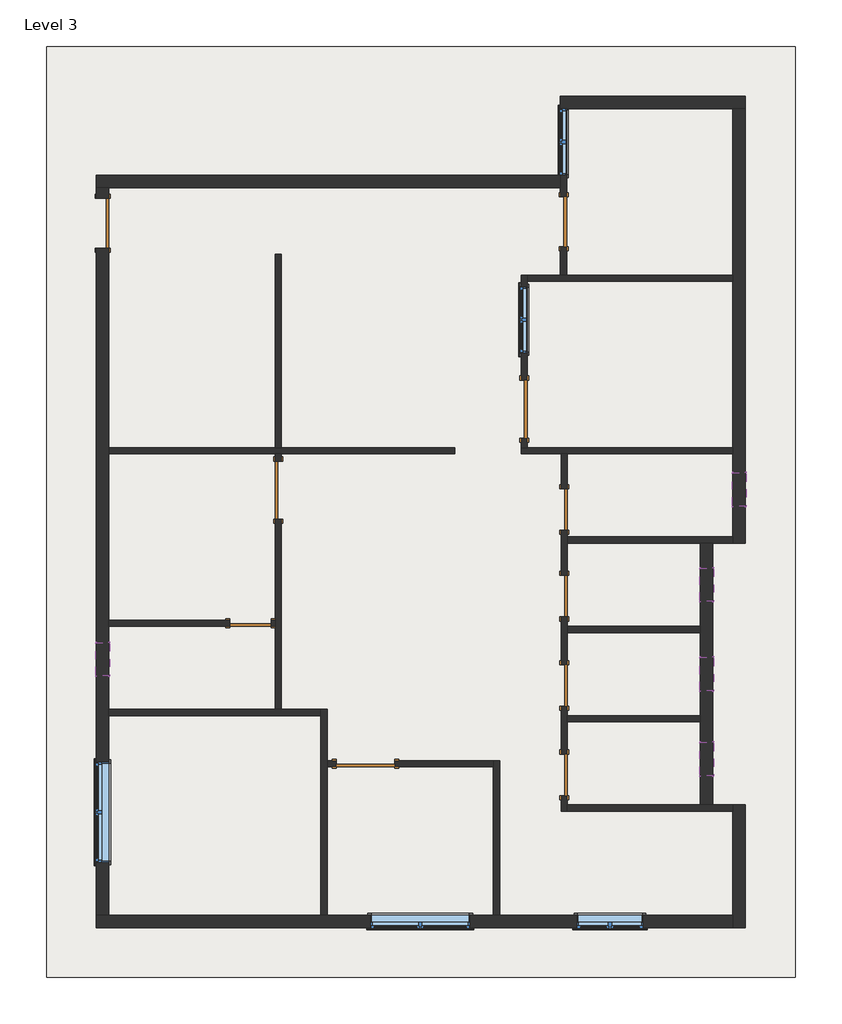
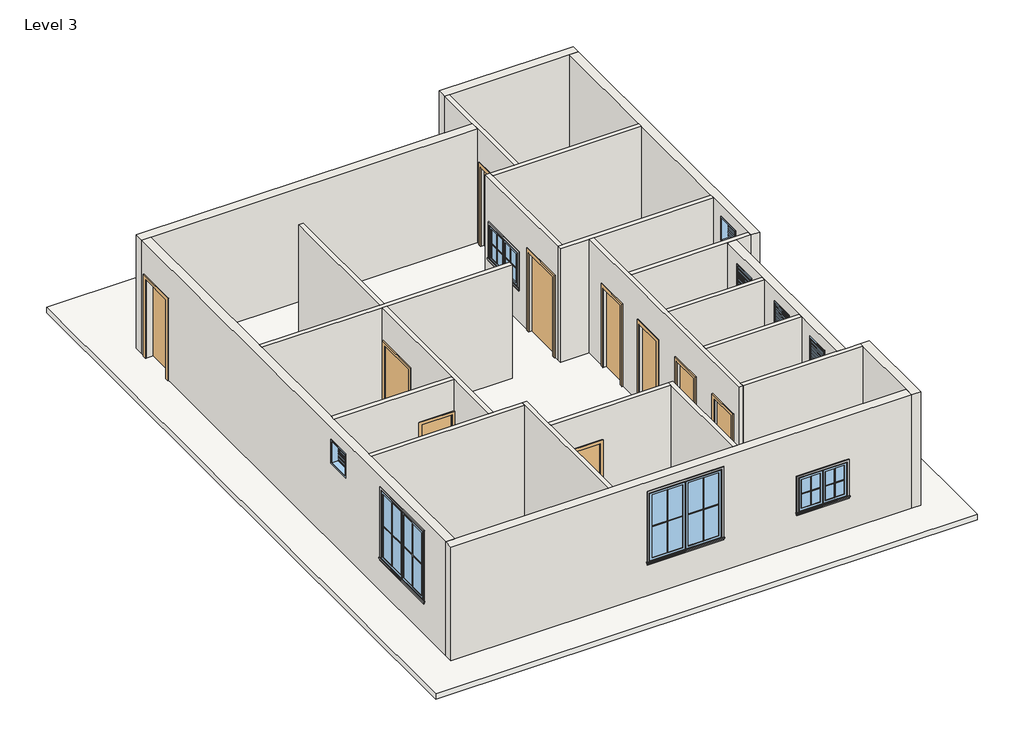
# One storey, incomplete: 23 walls, 20 proxies, 10 doors, 10 windows, 1 roof.
"""IFC4 building model written with IfcOpenShell, lengths in millimetres."""

from ifc_helpers import new_model, si_unit, frame, origin, place, context, project, spatial, polyline, outline, extrude, faceted_brep, transform, mapped, element, save
from components import muntin_pattern_2x2_muntin_pattern_2x2_0a037076, muntin_pattern_2x2_muntin_pattern_2x2_e6f69628, muntin_pattern_2x2_muntin_pattern_2x2_2357e71d, muntin_pattern_2x2_muntin_pattern_2x2_302d8f29, trim_window_exterior_flat_with_sill_b601e94a, trim_window_exterior_flat_with_sill_c4e67c73, trim_window_interior_flat_picture_frame_bfefb25c, trim_window_interior_flat_picture_frame_cf1733af, door_78caadf7, door_214872d5, single_flush_door_3_305aa2a5, single_flush_door_3_a90ba1ad, door_4c162e62, window_casement_double_win_4_c19c33cb, window_casement_double_win_4_2967420f, window_casement_double_win_6_ce442eab, window_f2d8fef0

model = new_model("IFC4")

# Units and contexts
model_context = context("Model", 3, world=origin())
ifc_project = project(units=[si_unit("LENGTHUNIT", "METRE", prefix="MILLI")], contexts=[model_context])

# Site, building, storey
site = spatial("IfcSite", under=ifc_project)
building = spatial("IfcBuilding", under=site)
storey = spatial("IfcBuildingStorey", under=building, Name="Level 3", Elevation=6248.4)

# Proxies
placement = place(None, origin())
muntin_pattern_2x2_muntin_pattern_2x2_shape = muntin_pattern_2x2_muntin_pattern_2x2_0a037076(model_context)
element("IfcBuildingElementProxy", 1, Name="Muntin Pattern_2x2 : Muntin Pattern_2x2", ObjectType="Muntin Pattern_2x2 : Muntin Pattern_2x2", at=placement, inside=storey, context=model_context, shape_type="MappedRepresentation", body=[
    mapped(muntin_pattern_2x2_muntin_pattern_2x2_shape, transform((-7058.058853, -4848.517381, 7232.65), x_axis=(0.0, 1.0, 0.0), y_axis=(-1.0, 0.0, 0.0), z_axis=(0.0, 0.0, 1.0))),
])
element("IfcBuildingElementProxy", 2, Name="Muntin Pattern_2x2 : Muntin Pattern_2x2", ObjectType="Muntin Pattern_2x2 : Muntin Pattern_2x2", at=placement, inside=storey, context=model_context, shape_type="MappedRepresentation", body=[
    mapped(muntin_pattern_2x2_muntin_pattern_2x2_shape, transform((-674.721353, -6497.929881, 7232.65), x_axis=(-1.0, 0.0, 0.0), y_axis=(0.0, -1.0, 0.0), z_axis=(0.0, 0.0, 1.0))),
])
muntin_pattern_2x2_muntin_pattern_2x2_2_shape = muntin_pattern_2x2_muntin_pattern_2x2_e6f69628(model_context)
element("IfcBuildingElementProxy", 3, Name="Muntin Pattern_2x2 : Muntin Pattern_2x2", ObjectType="Muntin Pattern_2x2 : Muntin Pattern_2x2", at=placement, inside=storey, context=model_context, shape_type="MappedRepresentation", body=[
    mapped(muntin_pattern_2x2_muntin_pattern_2x2_2_shape, transform((-7058.058853, -3937.292381, 7232.65), x_axis=(0.0, -1.0, 0.0), y_axis=(1.0, 0.0, 0.0), z_axis=(0.0, 0.0, 1.0))),
])
element("IfcBuildingElementProxy", 4, Name="Muntin Pattern_2x2 : Muntin Pattern_2x2", ObjectType="Muntin Pattern_2x2 : Muntin Pattern_2x2", at=placement, inside=storey, context=model_context, shape_type="MappedRepresentation", body=[
    mapped(muntin_pattern_2x2_muntin_pattern_2x2_2_shape, transform((-1585.946353, -6497.929881, 7232.65), x_axis=(1.0, 0.0, 0.0), y_axis=(0.0, 1.0, 0.0), z_axis=(0.0, 0.0, 1.0))),
])
muntin_pattern_2x2_muntin_pattern_2x2_3_shape = muntin_pattern_2x2_muntin_pattern_2x2_2357e71d(model_context)
element("IfcBuildingElementProxy", 5, Name="Muntin Pattern_2x2 : Muntin Pattern_2x2", ObjectType="Muntin Pattern_2x2 : Muntin Pattern_2x2", at=placement, inside=storey, context=model_context, shape_type="MappedRepresentation", body=[
    mapped(muntin_pattern_2x2_muntin_pattern_2x2_3_shape, transform((2652.678647, -6497.929881, 7232.65), x_axis=(-1.0, 0.0, 0.0), y_axis=(0.0, -1.0, 0.0), z_axis=(0.0, 0.0, 1.0))),
])
element("IfcBuildingElementProxy", 6, Name="Muntin Pattern_2x2 : Muntin Pattern_2x2", ObjectType="Muntin Pattern_2x2 : Muntin Pattern_2x2", at=placement, inside=storey, context=model_context, shape_type="MappedRepresentation", body=[
    mapped(muntin_pattern_2x2_muntin_pattern_2x2_3_shape, transform((727.041147, 4333.582619, 7232.65), x_axis=(0.0, 1.0, 0.0), y_axis=(-1.0, 0.0, 0.0), z_axis=(0.0, 0.0, 1.0))),
])
element("IfcBuildingElementProxy", 7, Name="Muntin Pattern_2x2 : Muntin Pattern_2x2", ObjectType="Muntin Pattern_2x2 : Muntin Pattern_2x2", at=placement, inside=storey, context=model_context, shape_type="MappedRepresentation", body=[
    mapped(muntin_pattern_2x2_muntin_pattern_2x2_3_shape, transform((1450.941147, 7591.132619, 7232.65), x_axis=(0.0, 1.0, 0.0), y_axis=(-1.0, 0.0, 0.0), z_axis=(0.0, 0.0, 1.0))),
])
muntin_pattern_2x2_muntin_pattern_2x2_4_shape = muntin_pattern_2x2_muntin_pattern_2x2_302d8f29(model_context)
element("IfcBuildingElementProxy", 8, Name="Muntin Pattern_2x2 : Muntin Pattern_2x2", ObjectType="Muntin Pattern_2x2 : Muntin Pattern_2x2", at=placement, inside=storey, context=model_context, shape_type="MappedRepresentation", body=[
    mapped(muntin_pattern_2x2_muntin_pattern_2x2_4_shape, transform((2046.253647, -6497.929881, 7232.65), x_axis=(1.0, 0.0, 0.0), y_axis=(0.0, 1.0, 0.0), z_axis=(0.0, 0.0, 1.0))),
])
element("IfcBuildingElementProxy", 9, Name="Muntin Pattern_2x2 : Muntin Pattern_2x2", ObjectType="Muntin Pattern_2x2 : Muntin Pattern_2x2", at=placement, inside=storey, context=model_context, shape_type="MappedRepresentation", body=[
    mapped(muntin_pattern_2x2_muntin_pattern_2x2_4_shape, transform((727.041147, 4940.007619, 7232.65), x_axis=(0.0, -1.0, 0.0), y_axis=(1.0, 0.0, 0.0), z_axis=(0.0, 0.0, 1.0))),
])
element("IfcBuildingElementProxy", 10, Name="Muntin Pattern_2x2 : Muntin Pattern_2x2", ObjectType="Muntin Pattern_2x2 : Muntin Pattern_2x2", at=placement, inside=storey, context=model_context, shape_type="MappedRepresentation", body=[
    mapped(muntin_pattern_2x2_muntin_pattern_2x2_4_shape, transform((1450.941147, 8197.557619, 7232.65), x_axis=(0.0, -1.0, 0.0), y_axis=(1.0, 0.0, 0.0), z_axis=(0.0, 0.0, 1.0))),
])
trim_window_exterior_flat_with_sill_shape = trim_window_exterior_flat_with_sill_b601e94a(model_context)
element("IfcBuildingElementProxy", 11, Name="Trim-Window-Exterior-Flat : with Sill", ObjectType="Trim-Window-Exterior-Flat : with Sill", at=placement, inside=storey, context=model_context, shape_type="MappedRepresentation", body=[
    mapped(trim_window_exterior_flat_with_sill_shape, transform((-7067.583853, -4392.904881, 8991.6), x_axis=(0.0, -1.0, 0.0), y_axis=(0.0, 0.0, 1.0), z_axis=(-1.0, 0.0, 0.0))),
])
element("IfcBuildingElementProxy", 12, Name="Trim-Window-Exterior-Flat : with Sill", ObjectType="Trim-Window-Exterior-Flat : with Sill", at=placement, inside=storey, context=model_context, shape_type="MappedRepresentation", body=[
    mapped(trim_window_exterior_flat_with_sill_shape, transform((-1130.333853, -6507.454881, 8991.6), x_axis=(1.0, 0.0, 0.0), y_axis=(0.0, 0.0, 1.0), z_axis=(0.0, -1.0, 0.0))),
])
trim_window_exterior_flat_with_sill_2_shape = trim_window_exterior_flat_with_sill_c4e67c73(model_context)
element("IfcBuildingElementProxy", 13, Name="Trim-Window-Exterior-Flat : with Sill", ObjectType="Trim-Window-Exterior-Flat : with Sill", at=placement, inside=storey, context=model_context, shape_type="MappedRepresentation", body=[
    mapped(trim_window_exterior_flat_with_sill_2_shape, transform((2349.466147, -6507.454881, 8077.2), x_axis=(1.0, 0.0, 0.0), y_axis=(0.0, 0.0, 1.0), z_axis=(0.0, -1.0, 0.0))),
])
element("IfcBuildingElementProxy", 14, Name="Trim-Window-Exterior-Flat : with Sill", ObjectType="Trim-Window-Exterior-Flat : with Sill", at=placement, inside=storey, context=model_context, shape_type="MappedRepresentation", body=[
    mapped(trim_window_exterior_flat_with_sill_2_shape, transform((717.516147, 4636.795119, 8077.2), x_axis=(0.0, -1.0, 0.0), y_axis=(0.0, 0.0, 1.0), z_axis=(-1.0, 0.0, 0.0))),
])
element("IfcBuildingElementProxy", 15, Name="Trim-Window-Exterior-Flat : with Sill", ObjectType="Trim-Window-Exterior-Flat : with Sill", at=placement, inside=storey, context=model_context, shape_type="MappedRepresentation", body=[
    mapped(trim_window_exterior_flat_with_sill_2_shape, transform((1441.416147, 7894.345119, 8077.2), x_axis=(0.0, -1.0, 0.0), y_axis=(0.0, 0.0, 1.0), z_axis=(-1.0, 0.0, 0.0))),
])
trim_window_interior_flat_picture_frame_shape = trim_window_interior_flat_picture_frame_bfefb25c(model_context)
element("IfcBuildingElementProxy", 16, Name="Trim-Window-Interior-Flat : Picture Frame", ObjectType="Trim-Window-Interior-Flat : Picture Frame", at=placement, inside=storey, context=model_context, shape_type="MappedRepresentation", body=[
    mapped(trim_window_interior_flat_picture_frame_shape, transform((-6838.983853, -4392.904881, 8991.6), x_axis=(0.0, 1.0, 0.0), y_axis=(0.0, 0.0, 1.0), z_axis=(1.0, 0.0, 0.0))),
])
element("IfcBuildingElementProxy", 17, Name="Trim-Window-Interior-Flat : Picture Frame", ObjectType="Trim-Window-Interior-Flat : Picture Frame", at=placement, inside=storey, context=model_context, shape_type="MappedRepresentation", body=[
    mapped(trim_window_interior_flat_picture_frame_shape, transform((-1130.333853, -6278.854881, 8991.6), x_axis=(-1.0, 0.0, 0.0), y_axis=(0.0, 0.0, 1.0), z_axis=(0.0, 1.0, 0.0))),
])
trim_window_interior_flat_picture_frame_2_shape = trim_window_interior_flat_picture_frame_cf1733af(model_context)
element("IfcBuildingElementProxy", 18, Name="Trim-Window-Interior-Flat : Picture Frame", ObjectType="Trim-Window-Interior-Flat : Picture Frame", at=placement, inside=storey, context=model_context, shape_type="MappedRepresentation", body=[
    mapped(trim_window_interior_flat_picture_frame_2_shape, transform((2349.466147, -6278.854881, 8077.2), x_axis=(-1.0, 0.0, 0.0), y_axis=(0.0, 0.0, 1.0), z_axis=(0.0, 1.0, 0.0))),
])
element("IfcBuildingElementProxy", 19, Name="Trim-Window-Interior-Flat : Picture Frame", ObjectType="Trim-Window-Interior-Flat : Picture Frame", at=placement, inside=storey, context=model_context, shape_type="MappedRepresentation", body=[
    mapped(trim_window_interior_flat_picture_frame_2_shape, transform((831.816147, 4636.795119, 8077.2), x_axis=(0.0, 1.0, 0.0), y_axis=(0.0, 0.0, 1.0), z_axis=(1.0, 0.0, 0.0))),
])
element("IfcBuildingElementProxy", 20, Name="Trim-Window-Interior-Flat : Picture Frame", ObjectType="Trim-Window-Interior-Flat : Picture Frame", at=placement, inside=storey, context=model_context, shape_type="MappedRepresentation", body=[
    mapped(trim_window_interior_flat_picture_frame_2_shape, transform((1555.716147, 7894.345119, 8077.2), x_axis=(0.0, 1.0, 0.0), y_axis=(0.0, 0.0, 1.0), z_axis=(1.0, 0.0, 0.0))),
])

# Doors
door_shape = door_78caadf7(model_context)
element("IfcDoor", 21, ObjectType="Single-Flush : 2'6\"", at=placement, inside=storey, context=model_context, shape_type="MappedRepresentation", body=[
    mapped(door_shape, transform((-4241.833853, -925.804881, 6248.4), x_axis=(1.0, 0.0, 0.0), y_axis=(0.0, 1.0, 0.0), z_axis=(0.0, 0.0, 1.0))),
])
door_2_shape = door_214872d5(model_context)
element("IfcDoor", 22, ObjectType="Single-Flush : 2'6\"", at=placement, inside=storey, context=model_context, shape_type="MappedRepresentation", body=[
    mapped(door_2_shape, transform((1511.266147, 1156.995119, 6248.4), x_axis=(0.0, -1.0, 0.0), y_axis=(1.0, 0.0, 0.0), z_axis=(0.0, 0.0, 1.0))),
])
element("IfcDoor", 23, ObjectType="Single-Flush : 2'6\"", at=placement, inside=storey, context=model_context, shape_type="MappedRepresentation", body=[
    mapped(door_2_shape, transform((1511.266147, -430.504881, 6248.4), x_axis=(0.0, -1.0, 0.0), y_axis=(1.0, 0.0, 0.0), z_axis=(0.0, 0.0, 1.0))),
])
element("IfcDoor", 24, ObjectType="Single-Flush : 2'6\"", at=placement, inside=storey, context=model_context, shape_type="MappedRepresentation", body=[
    mapped(door_2_shape, transform((1511.266147, -2068.804881, 6248.4), x_axis=(0.0, -1.0, 0.0), y_axis=(1.0, 0.0, 0.0), z_axis=(0.0, 0.0, 1.0))),
])
element("IfcDoor", 25, ObjectType="Single-Flush : 2'6\"", at=placement, inside=storey, context=model_context, shape_type="MappedRepresentation", body=[
    mapped(door_2_shape, transform((1511.266147, -3707.104881, 6248.4), x_axis=(0.0, -1.0, 0.0), y_axis=(1.0, 0.0, 0.0), z_axis=(0.0, 0.0, 1.0))),
])
single_flush_door_3_shape = single_flush_door_3_305aa2a5(model_context)
element("IfcDoor", 26, ObjectType="Single-Flush : DOOR 3'", at=placement, inside=storey, context=model_context, shape_type="MappedRepresentation", body=[
    mapped(single_flush_door_3_shape, transform((1498.566147, 6433.845119, 6248.4), x_axis=(0.0, 1.0, 0.0), y_axis=(-1.0, 0.0, 0.0), z_axis=(0.0, 0.0, 1.0))),
])
single_flush_door_3_2_shape = single_flush_door_3_a90ba1ad(model_context)
element("IfcDoor", 27, ObjectType="Single-Flush : DOOR 3'", at=placement, inside=storey, context=model_context, shape_type="MappedRepresentation", body=[
    mapped(single_flush_door_3_2_shape, transform((-6953.283853, 6408.445119, 6248.4), x_axis=(0.0, 1.0, 0.0), y_axis=(-1.0, 0.0, 0.0), z_axis=(0.0, 0.0, 1.0))),
])
door_3_shape = door_4c162e62(model_context)
element("IfcDoor", 28, ObjectType="Single-Flush : DOOR 3'6\"", at=placement, inside=storey, context=model_context, shape_type="MappedRepresentation", body=[
    mapped(door_3_shape, transform((-3733.833853, 1512.595119, 6248.4), x_axis=(0.0, 1.0, 0.0), y_axis=(-1.0, 0.0, 0.0), z_axis=(0.0, 0.0, 1.0))),
])
element("IfcDoor", 29, ObjectType="Single-Flush : DOOR 3'6\"", at=placement, inside=storey, context=model_context, shape_type="MappedRepresentation", body=[
    mapped(door_3_shape, transform((774.666147, 2998.495119, 6248.4), x_axis=(0.0, -1.0, 0.0), y_axis=(1.0, 0.0, 0.0), z_axis=(0.0, 0.0, 1.0))),
])
element("IfcDoor", 30, ObjectType="Single-Flush : DOOR 3'6\"", at=placement, inside=storey, context=model_context, shape_type="MappedRepresentation", body=[
    mapped(door_3_shape, transform((-2133.633853, -3503.904881, 6248.4), x_axis=(-1.0, 0.0, 0.0), y_axis=(0.0, -1.0, 0.0), z_axis=(0.0, 0.0, 1.0))),
])

# Roof
element("IfcRoof", 31, ObjectType="Generic - 12\"", at=placement, inside=storey, context=model_context, shape_type="SweptSolid", body=[
    extrude(outline(polyline([(-7981.983853, 9646.945119), (5746.716147, 9646.945119), (5746.716147, -7421.854881), (-7981.983853, -7421.854881), (-7981.983853, 9646.945119)])), frame((0.0, 0.0, 6096.0), z_axis=(0.0, 0.0, 1.0), x_axis=(1.0, 0.0, 0.0)), (0.0, 0.0, 1.0), 152.4),
])

# Walls
element("IfcWall", 32, ObjectType="WALL 4.5\"", at=placement, inside=storey, context=model_context, shape_type="Brep", body=[
    faceted_brep([(-6838.983853, 2179.345119, 6248.4), (-3790.983853, 2179.345119, 6248.4), (-3676.683853, 2179.345119, 6248.4), (-501.683853, 2179.345119, 6248.4), (-501.683853, 2179.345119, 9296.4), (-3676.683853, 2179.345119, 9296.4), (-3790.983853, 2179.345119, 9296.4), (-6838.983853, 2179.345119, 9296.4), (-6838.983853, 2293.645119, 6248.4), (-6838.983853, 2293.645119, 9296.4), (-3790.983853, 2293.645119, 9296.4), (-3676.683853, 2293.645119, 9296.4), (-501.683853, 2293.645119, 9296.4), (-501.683853, 2293.645119, 6248.4), (-3676.683853, 2293.645119, 6248.4), (-3790.983853, 2293.645119, 6248.4)], [[[0, 1, 2, 3, 4, 5, 6, 7]], [[8, 9, 10, 11, 12, 13, 14, 15]], [[3, 2, 1, 0, 8, 15, 14, 13]], [[4, 3, 13, 12]], [[0, 7, 9, 8]], [[7, 6, 5, 4, 12, 11, 10, 9]]]),
])
element("IfcWall", 33, ObjectType="WALL 4.5\"", at=placement, inside=storey, context=model_context, shape_type="Brep", body=[
    faceted_brep([(-2838.483853, -6278.854881, 6248.4), (-2838.483853, -3561.054881, 6248.4), (-2838.483853, -3446.754881, 6248.4), (-2838.483853, -2506.954881, 6248.4), (-2838.483853, -2506.954881, 9296.4), (-2838.483853, -3446.754881, 9296.4), (-2838.483853, -3561.054881, 9296.4), (-2838.483853, -6278.854881, 9296.4), (-2952.783853, -6278.854881, 6248.4), (-2952.783853, -6278.854881, 9296.4), (-2952.783853, -2621.254881, 9296.4), (-2952.783853, -2506.954881, 9296.4), (-2952.783853, -2506.954881, 6248.4), (-2952.783853, -2621.254881, 6248.4)], [[[0, 1, 2, 3, 4, 5, 6, 7]], [[8, 9, 10, 11, 12, 13]], [[3, 2, 1, 0, 8, 13, 12]], [[0, 7, 9, 8]], [[4, 3, 12, 11]], [[7, 6, 5, 4, 11, 10, 9]]]),
])
element("IfcWall", 34, ObjectType="WALL 4.5\"", at=placement, inside=storey, context=model_context, shape_type="Brep", body=[
    faceted_brep([(-2952.783853, -2506.954881, 6248.4), (-3676.683853, -2506.954881, 6248.4), (-3790.983853, -2506.954881, 6248.4), (-6838.983853, -2506.954881, 6248.4), (-6838.983853, -2506.954881, 9296.4), (-3790.983853, -2506.954881, 9296.4), (-3676.683853, -2506.954881, 9296.4), (-2952.783853, -2506.954881, 9296.4), (-2952.783853, -2621.254881, 6248.4), (-2952.783853, -2621.254881, 9296.4), (-6838.983853, -2621.254881, 9296.4), (-6838.983853, -2621.254881, 6248.4)], [[[0, 1, 2, 3, 4, 5, 6, 7]], [[8, 9, 10, 11]], [[3, 2, 1, 0, 8, 11]], [[0, 7, 9, 8]], [[4, 3, 11, 10]], [[7, 6, 5, 4, 10, 9]]]),
])
element("IfcWall", 35, ObjectType="WALL 4.5\"", at=placement, inside=storey, context=model_context, shape_type="SweptSolid", body=[
    extrude(outline(polyline([(8382.0, -3860.833853), (6248.4, -3860.833853), (6248.4, -3790.983853), (9296.4, -3790.983853), (9296.4, -6838.983853), (6248.4, -6838.983853), (6248.4, -4622.833853), (8382.0, -4622.833853), (8382.0, -3860.833853)])), frame((0.0, -982.954881, 0.0), z_axis=(0.0, 1.0, 0.0), x_axis=(0.0, 0.0, 1.0)), (0.0, 0.0, 1.0), 114.3),
])
element("IfcWall", 36, ObjectType="WALL 4.5\"", at=placement, inside=storey, context=model_context, shape_type="Brep", body=[
    faceted_brep([(-3676.683853, 5836.945119, 6248.4), (-3676.683853, 5836.945119, 9296.4), (-3676.683853, 2293.645119, 9296.4), (-3676.683853, 2293.645119, 6248.4), (-3790.983853, 5836.945119, 9296.4), (-3790.983853, 5836.945119, 6248.4), (-3790.983853, 2293.645119, 6248.4), (-3790.983853, 2293.645119, 9296.4)], [[[0, 1, 2, 3]], [[4, 5, 6, 7]], [[5, 0, 3, 6]], [[1, 0, 5, 4]], [[3, 2, 7, 6]], [[1, 4, 7, 2]]]),
    faceted_brep([(-3676.683853, -2506.954881, 9296.4), (-3676.683853, -2506.954881, 6248.4), (-3676.683853, 979.195119, 6248.4), (-3676.683853, 979.195119, 8382.0), (-3676.683853, 2045.995119, 8382.0), (-3676.683853, 2045.995119, 6248.4), (-3676.683853, 2179.345119, 6248.4), (-3676.683853, 2179.345119, 9296.4), (-3790.983853, -2506.954881, 6248.4), (-3790.983853, -2506.954881, 9296.4), (-3790.983853, -982.954881, 9296.4), (-3790.983853, -868.654881, 9296.4), (-3790.983853, 2179.345119, 9296.4), (-3790.983853, 2179.345119, 6248.4), (-3790.983853, 2045.995119, 6248.4), (-3790.983853, 2045.995119, 8382.0), (-3790.983853, 979.195119, 8382.0), (-3790.983853, 979.195119, 6248.4), (-3790.983853, -868.654881, 6248.4), (-3790.983853, -982.954881, 6248.4)], [[[0, 1, 2, 3, 4, 5, 6, 7]], [[8, 9, 10, 11, 12, 13, 14, 15, 16, 17, 18, 19]], [[1, 8, 19, 18, 17, 2]], [[5, 14, 13, 6]], [[1, 0, 9, 8]], [[7, 6, 13, 12]], [[15, 14, 5, 4]], [[16, 15, 4, 3]], [[17, 16, 3, 2]], [[9, 0, 7, 12, 11, 10]]]),
])
element("IfcWall", 37, ObjectType="WALL 4.5\"", at=placement, inside=storey, context=model_context, shape_type="Brep", body=[
    faceted_brep([(4603.716147, 2293.645119, 6248.4), (831.816147, 2293.645119, 6248.4), (717.516147, 2293.645119, 6248.4), (717.516147, 2293.645119, 9296.4), (831.816147, 2293.645119, 9296.4), (4603.716147, 2293.645119, 9296.4), (4603.716147, 2179.345119, 6248.4), (4603.716147, 2179.345119, 9296.4), (1568.416147, 2179.345119, 9296.4), (1454.116147, 2179.345119, 9296.4), (717.516147, 2179.345119, 9296.4), (717.516147, 2179.345119, 6248.4), (1454.116147, 2179.345119, 6248.4), (1568.416147, 2179.345119, 6248.4)], [[[0, 1, 2, 3, 4, 5]], [[6, 7, 8, 9, 10, 11, 12, 13]], [[2, 1, 0, 6, 13, 12, 11]], [[0, 5, 7, 6]], [[3, 2, 11, 10]], [[5, 4, 3, 10, 9, 8, 7]]]),
])
element("IfcWall", 38, ObjectType="WALL 4.5\"", at=placement, inside=storey, context=model_context, shape_type="Brep", body=[
    faceted_brep([(831.816147, 2293.645119, 6248.4), (831.816147, 2465.095119, 6248.4), (831.816147, 2465.095119, 8382.0), (831.816147, 3531.895119, 8382.0), (831.816147, 3531.895119, 6248.4), (831.816147, 5341.645119, 6248.4), (831.816147, 5455.945119, 6248.4), (831.816147, 5455.945119, 9296.4), (831.816147, 5341.645119, 9296.4), (831.816147, 2293.645119, 9296.4), (831.816147, 5246.395119, 8077.2), (831.816147, 5246.395119, 7162.8), (831.816147, 4027.195119, 7162.8), (831.816147, 4027.195119, 8077.2), (717.516147, 2465.095119, 8382.0), (717.516147, 2465.095119, 6248.4), (717.516147, 2293.645119, 6248.4), (717.516147, 2293.645119, 9296.4), (717.516147, 5455.945119, 9296.4), (717.516147, 5455.945119, 6248.4), (717.516147, 3531.895119, 6248.4), (717.516147, 3531.895119, 8382.0), (717.516147, 5246.395119, 8077.2), (717.516147, 4027.195119, 8077.2), (717.516147, 4027.195119, 7162.8), (717.516147, 5246.395119, 7162.8)], [[[0, 1, 2, 3, 4, 5, 6, 7, 8, 9], [10, 11, 12, 13]], [[14, 15, 16, 17, 18, 19, 20, 21], [22, 23, 24, 25]], [[20, 19, 6, 5, 4]], [[16, 15, 1, 0]], [[0, 9, 17, 16]], [[7, 6, 19, 18]], [[11, 10, 22, 25]], [[12, 11, 25, 24]], [[13, 12, 24, 23]], [[10, 13, 23, 22]], [[2, 1, 15, 14]], [[3, 2, 14, 21]], [[4, 3, 21, 20]], [[9, 8, 7, 18, 17]]]),
])
element("IfcWall", 39, ObjectType="WALL 4.5\"", at=placement, inside=storey, context=model_context, shape_type="Brep", body=[
    faceted_brep([(831.816147, 5341.645119, 6248.4), (4603.716147, 5341.645119, 6248.4), (4603.716147, 5341.645119, 9296.4), (831.816147, 5341.645119, 9296.4), (831.816147, 5455.945119, 6248.4), (831.816147, 5455.945119, 9296.4), (1441.416147, 5455.945119, 9296.4), (1555.716147, 5455.945119, 9296.4), (4603.716147, 5455.945119, 9296.4), (4603.716147, 5455.945119, 6248.4), (1555.716147, 5455.945119, 6248.4), (1441.416147, 5455.945119, 6248.4)], [[[0, 1, 2, 3]], [[4, 5, 6, 7, 8, 9, 10, 11]], [[1, 0, 4, 11, 10, 9]], [[0, 3, 5, 4]], [[2, 1, 9, 8]], [[3, 2, 8, 7, 6, 5]]]),
])
element("IfcWall", 40, ObjectType="WALL 4.5\"", at=placement, inside=storey, context=model_context, shape_type="Brep", body=[
    faceted_brep([(1555.716147, 6891.045119, 8382.0), (1555.716147, 6891.045119, 6248.4), (1555.716147, 8503.945119, 6248.4), (1555.716147, 8503.945119, 7162.8), (1555.716147, 7284.745119, 7162.8), (1555.716147, 7284.745119, 8077.2), (1555.716147, 8503.945119, 8077.2), (1555.716147, 8503.945119, 9296.4), (1555.716147, 5455.945119, 9296.4), (1555.716147, 5455.945119, 6248.4), (1555.716147, 5976.645119, 6248.4), (1555.716147, 5976.645119, 8382.0), (1441.416147, 8503.945119, 6248.4), (1441.416147, 7284.745119, 6248.4), (1441.416147, 7056.145119, 6248.4), (1441.416147, 6891.045119, 6248.4), (1441.416147, 6891.045119, 8382.0), (1441.416147, 5976.645119, 8382.0), (1441.416147, 5976.645119, 6248.4), (1441.416147, 5455.945119, 6248.4), (1441.416147, 5455.945119, 9296.4), (1441.416147, 7056.145119, 9296.4), (1441.416147, 7284.745119, 9296.4), (1441.416147, 8503.945119, 9296.4), (1441.416147, 8503.945119, 8077.2), (1441.416147, 7284.745119, 8077.2), (1441.416147, 7284.745119, 7162.8), (1441.416147, 8503.945119, 7162.8)], [[[0, 1, 2, 3, 4, 5, 6, 7, 8, 9, 10, 11]], [[12, 13, 14, 15, 16, 17, 18, 19, 20, 21, 22, 23, 24, 25, 26, 27]], [[10, 9, 19, 18]], [[2, 1, 15, 14, 13, 12]], [[24, 23, 7, 6]], [[12, 27, 3, 2]], [[9, 8, 20, 19]], [[4, 3, 27, 26]], [[5, 4, 26, 25]], [[6, 5, 25, 24]], [[16, 15, 1, 0]], [[17, 16, 0, 11]], [[18, 17, 11, 10]], [[8, 7, 23, 22, 21, 20]]]),
])
element("IfcWall", 41, ObjectType="WALL 4.5\"", at=placement, inside=storey, context=model_context, shape_type="Brep", body=[
    faceted_brep([(4603.716147, 655.345119, 6248.4), (1568.416147, 655.345119, 6248.4), (1568.416147, 655.345119, 9296.4), (4603.716147, 655.345119, 9296.4), (4603.716147, 541.045119, 6248.4), (4603.716147, 541.045119, 9296.4), (4235.416147, 541.045119, 9296.4), (4006.816147, 541.045119, 9296.4), (1568.416147, 541.045119, 9296.4), (1568.416147, 541.045119, 6248.4), (4006.816147, 541.045119, 6248.4), (4235.416147, 541.045119, 6248.4)], [[[0, 1, 2, 3]], [[4, 5, 6, 7, 8, 9, 10, 11]], [[1, 0, 4, 11, 10, 9]], [[0, 3, 5, 4]], [[2, 1, 9, 8]], [[3, 2, 8, 7, 6, 5]]]),
])
element("IfcWall", 42, ObjectType="WALL 4.5\"", at=placement, inside=storey, context=model_context, shape_type="Brep", body=[
    faceted_brep([(1454.116147, -4088.104881, 8382.0), (1454.116147, -4088.104881, 6248.4), (1454.116147, -4373.854881, 6248.4), (1454.116147, -4373.854881, 9296.4), (1454.116147, 2179.345119, 9296.4), (1454.116147, 2179.345119, 6248.4), (1454.116147, 1537.995119, 6248.4), (1454.116147, 1537.995119, 8382.0), (1454.116147, 775.995119, 8382.0), (1454.116147, 775.995119, 6248.4), (1454.116147, -49.504881, 6248.4), (1454.116147, -49.504881, 8382.0), (1454.116147, -811.504881, 8382.0), (1454.116147, -811.504881, 6248.4), (1454.116147, -1687.804881, 6248.4), (1454.116147, -1687.804881, 8382.0), (1454.116147, -2449.804881, 8382.0), (1454.116147, -2449.804881, 6248.4), (1454.116147, -3326.104881, 6248.4), (1454.116147, -3326.104881, 8382.0), (1568.416147, -4373.854881, 6248.4), (1568.416147, -4259.554881, 6248.4), (1568.416147, -4088.104881, 6248.4), (1568.416147, -4088.104881, 8382.0), (1568.416147, -3326.104881, 8382.0), (1568.416147, -3326.104881, 6248.4), (1568.416147, -2735.554881, 6248.4), (1568.416147, -2621.254881, 6248.4), (1568.416147, -2449.804881, 6248.4), (1568.416147, -2449.804881, 8382.0), (1568.416147, -1687.804881, 8382.0), (1568.416147, -1687.804881, 6248.4), (1568.416147, -1097.254881, 6248.4), (1568.416147, -982.954881, 6248.4), (1568.416147, -811.504881, 6248.4), (1568.416147, -811.504881, 8382.0), (1568.416147, -49.504881, 8382.0), (1568.416147, -49.504881, 6248.4), (1568.416147, 541.045119, 6248.4), (1568.416147, 655.345119, 6248.4), (1568.416147, 775.995119, 6248.4), (1568.416147, 775.995119, 8382.0), (1568.416147, 1537.995119, 8382.0), (1568.416147, 1537.995119, 6248.4), (1568.416147, 2179.345119, 6248.4), (1568.416147, 2179.345119, 9296.4), (1568.416147, 655.345119, 9296.4), (1568.416147, 541.045119, 9296.4), (1568.416147, -982.954881, 9296.4), (1568.416147, -1097.254881, 9296.4), (1568.416147, -2621.254881, 9296.4), (1568.416147, -2735.554881, 9296.4), (1568.416147, -4259.554881, 9296.4), (1568.416147, -4373.854881, 9296.4)], [[[0, 1, 2, 3, 4, 5, 6, 7, 8, 9, 10, 11, 12, 13, 14, 15, 16, 17, 18, 19]], [[20, 21, 22, 23, 24, 25, 26, 27, 28, 29, 30, 31, 32, 33, 34, 35, 36, 37, 38, 39, 40, 41, 42, 43, 44, 45, 46, 47, 48, 49, 50, 51, 52, 53]], [[6, 5, 44, 43]], [[10, 9, 40, 39, 38, 37]], [[14, 13, 34, 33, 32, 31]], [[18, 17, 28, 27, 26, 25]], [[2, 1, 22, 21, 20]], [[5, 4, 45, 44]], [[3, 2, 20, 53]], [[41, 40, 9, 8]], [[42, 41, 8, 7]], [[43, 42, 7, 6]], [[35, 34, 13, 12]], [[36, 35, 12, 11]], [[37, 36, 11, 10]], [[29, 28, 17, 16]], [[30, 29, 16, 15]], [[31, 30, 15, 14]], [[23, 22, 1, 0]], [[24, 23, 0, 19]], [[25, 24, 19, 18]], [[4, 3, 53, 52, 51, 50, 49, 48, 47, 46, 45]]]),
])
element("IfcWall", 43, ObjectType="WALL 4.5\"", at=placement, inside=storey, context=model_context, shape_type="Brep", body=[
    faceted_brep([(1568.416147, -4373.854881, 6248.4), (4603.716147, -4373.854881, 6248.4), (4603.716147, -4373.854881, 9296.4), (1568.416147, -4373.854881, 9296.4), (1568.416147, -4259.554881, 6248.4), (1568.416147, -4259.554881, 9296.4), (4006.816147, -4259.554881, 9296.4), (4235.416147, -4259.554881, 9296.4), (4603.716147, -4259.554881, 9296.4), (4603.716147, -4259.554881, 6248.4), (4235.416147, -4259.554881, 6248.4), (4006.816147, -4259.554881, 6248.4)], [[[0, 1, 2, 3]], [[4, 5, 6, 7, 8, 9, 10, 11]], [[1, 0, 4, 11, 10, 9]], [[0, 3, 5, 4]], [[2, 1, 9, 8]], [[3, 2, 8, 7, 6, 5]]]),
])
element("IfcWall", 44, ObjectType="WALL 4.5\"", at=placement, inside=storey, context=model_context, shape_type="SweptSolid", body=[
    extrude(outline(polyline([(4006.816147, -2735.554881), (1568.416147, -2735.554881), (1568.416147, -2621.254881), (4006.816147, -2621.254881), (4006.816147, -2735.554881)])), frame((0.0, 0.0, 6248.4), z_axis=(0.0, 0.0, 1.0), x_axis=(1.0, 0.0, 0.0)), (0.0, 0.0, 1.0), 3048.0),
])
element("IfcWall", 45, ObjectType="WALL 4.5\"", at=placement, inside=storey, context=model_context, shape_type="SweptSolid", body=[
    extrude(outline(polyline([(4006.816147, -1097.254881), (1568.416147, -1097.254881), (1568.416147, -982.954881), (4006.816147, -982.954881), (4006.816147, -1097.254881)])), frame((0.0, 0.0, 6248.4), z_axis=(0.0, 0.0, 1.0), x_axis=(1.0, 0.0, 0.0)), (0.0, 0.0, 1.0), 3048.0),
])
element("IfcWall", 46, ObjectType="WALL 4.5\"", at=placement, inside=storey, context=model_context, shape_type="Brep", body=[
    faceted_brep([(323.816147, -6278.854881, 6248.4), (323.816147, -3446.754881, 6248.4), (323.816147, -3446.754881, 9296.4), (323.816147, -6278.854881, 9296.4), (209.516147, -6278.854881, 6248.4), (209.516147, -6278.854881, 9296.4), (209.516147, -3561.054881, 9296.4), (209.516147, -3446.754881, 9296.4), (209.516147, -3446.754881, 6248.4), (209.516147, -3561.054881, 6248.4)], [[[0, 1, 2, 3]], [[4, 5, 6, 7, 8, 9]], [[1, 0, 4, 9, 8]], [[0, 3, 5, 4]], [[2, 1, 8, 7]], [[3, 2, 7, 6, 5]]]),
])
element("IfcWall", 47, ObjectType="WALL 4.5\"", at=placement, inside=storey, context=model_context, shape_type="SweptSolid", body=[
    extrude(outline(polyline([(6248.4, -2838.483853), (6248.4, -2667.033853), (8382.0, -2667.033853), (8382.0, -1600.233853), (6248.4, -1600.233853), (6248.4, 209.516147), (9296.4, 209.516147), (9296.4, -2838.483853), (6248.4, -2838.483853)])), frame((0.0, -3561.054881, 0.0), z_axis=(0.0, 1.0, 0.0), x_axis=(0.0, 0.0, 1.0)), (0.0, 0.0, 1.0), 114.3),
])
element("IfcWall", 48, ObjectType="WALL 9\"", at=placement, inside=storey, context=model_context, shape_type="Brep", body=[
    faceted_brep([(-7067.583853, 7056.145119, 6248.4), (-6838.983853, 7056.145119, 6248.4), (1441.416147, 7056.145119, 6248.4), (1441.416147, 7056.145119, 9296.4), (-6838.983853, 7056.145119, 9296.4), (-7067.583853, 7056.145119, 9296.4), (-7067.583853, 7284.745119, 6248.4), (-7067.583853, 7284.745119, 9296.4), (1441.416147, 7284.745119, 9296.4), (1441.416147, 7284.745119, 6248.4)], [[[0, 1, 2, 3, 4, 5]], [[6, 7, 8, 9]], [[2, 1, 0, 6, 9]], [[0, 5, 7, 6]], [[3, 2, 9, 8]], [[5, 4, 3, 8, 7]]]),
])
element("IfcWall", 49, ObjectType="WALL 9\"", at=placement, inside=storey, context=model_context, shape_type="Brep", body=[
    faceted_brep([(1441.416147, 8503.945119, 6248.4), (1555.716147, 8503.945119, 6248.4), (4603.716147, 8503.945119, 6248.4), (4832.316147, 8503.945119, 6248.4), (4832.316147, 8503.945119, 9296.4), (4603.716147, 8503.945119, 9296.4), (1555.716147, 8503.945119, 9296.4), (1441.416147, 8503.945119, 9296.4), (1441.416147, 8503.945119, 8077.2), (1441.416147, 8503.945119, 7162.8), (1441.416147, 8732.545119, 6248.4), (1441.416147, 8732.545119, 9296.4), (4832.316147, 8732.545119, 9296.4), (4832.316147, 8732.545119, 6248.4)], [[[0, 1, 2, 3, 4, 5, 6, 7, 8, 9]], [[10, 11, 12, 13]], [[3, 2, 1, 0, 10, 13]], [[4, 3, 13, 12]], [[0, 9, 8, 7, 11, 10]], [[7, 6, 5, 4, 12, 11]]]),
])
element("IfcWall", 50, ObjectType="WALL 9\"", at=placement, inside=storey, context=model_context, shape_type="Brep", body=[
    faceted_brep([(4603.716147, 8503.945119, 6248.4), (4603.716147, 5455.945119, 6248.4), (4603.716147, 5341.645119, 6248.4), (4603.716147, 2293.645119, 6248.4), (4603.716147, 2179.345119, 6248.4), (4603.716147, 655.345119, 6248.4), (4603.716147, 541.045119, 6248.4), (4603.716147, 541.045119, 9296.4), (4603.716147, 655.345119, 9296.4), (4603.716147, 2179.345119, 9296.4), (4603.716147, 2293.645119, 9296.4), (4603.716147, 5341.645119, 9296.4), (4603.716147, 5455.945119, 9296.4), (4603.716147, 8503.945119, 9296.4), (4603.716147, 1830.095119, 8991.6), (4603.716147, 1220.495119, 8991.6), (4603.716147, 1220.495119, 8382.0), (4603.716147, 1830.095119, 8382.0), (4832.316147, 8503.945119, 6248.4), (4832.316147, 8503.945119, 9296.4), (4832.316147, 541.045119, 9296.4), (4832.316147, 541.045119, 6248.4), (4832.316147, 1830.095119, 8991.6), (4832.316147, 1830.095119, 8382.0), (4832.316147, 1220.495119, 8382.0), (4832.316147, 1220.495119, 8991.6)], [[[0, 1, 2, 3, 4, 5, 6, 7, 8, 9, 10, 11, 12, 13], [14, 15, 16, 17]], [[18, 19, 20, 21], [22, 23, 24, 25]], [[6, 5, 4, 3, 2, 1, 0, 18, 21]], [[0, 13, 19, 18]], [[7, 6, 21, 20]], [[23, 22, 14, 17]], [[24, 23, 17, 16]], [[25, 24, 16, 15]], [[22, 25, 15, 14]], [[13, 12, 11, 10, 9, 8, 7, 20, 19]]]),
])
element("IfcWall", 51, ObjectType="WALL 9\"", at=placement, inside=storey, context=model_context, shape_type="Brep", body=[
    faceted_brep([(4006.816147, 541.045119, 6248.4), (4006.816147, -982.954881, 6248.4), (4006.816147, -1097.254881, 6248.4), (4006.816147, -2621.254881, 6248.4), (4006.816147, -2735.554881, 6248.4), (4006.816147, -4259.554881, 6248.4), (4006.816147, -4259.554881, 9296.4), (4006.816147, -2735.554881, 9296.4), (4006.816147, -2621.254881, 9296.4), (4006.816147, -1097.254881, 9296.4), (4006.816147, -982.954881, 9296.4), (4006.816147, 541.045119, 9296.4), (4006.816147, -525.754881, 8991.6), (4006.816147, -525.754881, 8382.0), (4006.816147, 83.845119, 8382.0), (4006.816147, 83.845119, 8991.6), (4006.816147, -2164.054881, 8991.6), (4006.816147, -2164.054881, 8382.0), (4006.816147, -1554.454881, 8382.0), (4006.816147, -1554.454881, 8991.6), (4006.816147, -3719.804881, 8991.6), (4006.816147, -3719.804881, 8382.0), (4006.816147, -3110.204881, 8382.0), (4006.816147, -3110.204881, 8991.6), (4235.416147, 541.045119, 6248.4), (4235.416147, 541.045119, 9296.4), (4235.416147, -4259.554881, 9296.4), (4235.416147, -4259.554881, 6248.4), (4235.416147, -525.754881, 8991.6), (4235.416147, 83.845119, 8991.6), (4235.416147, 83.845119, 8382.0), (4235.416147, -525.754881, 8382.0), (4235.416147, -2164.054881, 8991.6), (4235.416147, -1554.454881, 8991.6), (4235.416147, -1554.454881, 8382.0), (4235.416147, -2164.054881, 8382.0), (4235.416147, -3719.804881, 8991.6), (4235.416147, -3110.204881, 8991.6), (4235.416147, -3110.204881, 8382.0), (4235.416147, -3719.804881, 8382.0)], [[[0, 1, 2, 3, 4, 5, 6, 7, 8, 9, 10, 11], [12, 13, 14, 15], [16, 17, 18, 19], [20, 21, 22, 23]], [[24, 25, 26, 27], [28, 29, 30, 31], [32, 33, 34, 35], [36, 37, 38, 39]], [[5, 4, 3, 2, 1, 0, 24, 27]], [[0, 11, 25, 24]], [[6, 5, 27, 26]], [[13, 12, 28, 31]], [[14, 13, 31, 30]], [[15, 14, 30, 29]], [[12, 15, 29, 28]], [[17, 16, 32, 35]], [[18, 17, 35, 34]], [[19, 18, 34, 33]], [[16, 19, 33, 32]], [[21, 20, 36, 39]], [[22, 21, 39, 38]], [[23, 22, 38, 37]], [[20, 23, 37, 36]], [[11, 10, 9, 8, 7, 6, 26, 25]]]),
])
element("IfcWall", 52, ObjectType="WALL 9\"", at=placement, inside=storey, context=model_context, shape_type="Brep", body=[
    faceted_brep([(4603.716147, -4259.554881, 6248.4), (4603.716147, -4373.854881, 6248.4), (4603.716147, -6278.854881, 6248.4), (4603.716147, -6507.454881, 6248.4), (4603.716147, -6507.454881, 9296.4), (4603.716147, -6278.854881, 9296.4), (4603.716147, -4373.854881, 9296.4), (4603.716147, -4259.554881, 9296.4), (4832.316147, -4259.554881, 6248.4), (4832.316147, -4259.554881, 9296.4), (4832.316147, -6507.454881, 9296.4), (4832.316147, -6507.454881, 6248.4)], [[[0, 1, 2, 3, 4, 5, 6, 7]], [[8, 9, 10, 11]], [[3, 2, 1, 0, 8, 11]], [[4, 3, 11, 10]], [[0, 7, 9, 8]], [[7, 6, 5, 4, 10, 9]]]),
])
element("IfcWall", 53, ObjectType="WALL 9\"", at=placement, inside=storey, context=model_context, shape_type="Brep", body=[
    faceted_brep([(4603.716147, -6278.854881, 6248.4), (323.816147, -6278.854881, 6248.4), (209.516147, -6278.854881, 6248.4), (-2838.483853, -6278.854881, 6248.4), (-2952.783853, -6278.854881, 6248.4), (-6838.983853, -6278.854881, 6248.4), (-7067.583853, -6278.854881, 6248.4), (-7067.583853, -6278.854881, 9296.4), (-6838.983853, -6278.854881, 9296.4), (-2952.783853, -6278.854881, 9296.4), (-2838.483853, -6278.854881, 9296.4), (209.516147, -6278.854881, 9296.4), (323.816147, -6278.854881, 9296.4), (4603.716147, -6278.854881, 9296.4), (-2044.733853, -6278.854881, 8991.6), (-2044.733853, -6278.854881, 7162.8), (-215.933853, -6278.854881, 7162.8), (-215.933853, -6278.854881, 8991.6), (1739.866147, -6278.854881, 8077.2), (1739.866147, -6278.854881, 7162.8), (2959.066147, -6278.854881, 7162.8), (2959.066147, -6278.854881, 8077.2), (4603.716147, -6507.454881, 6248.4), (4603.716147, -6507.454881, 9296.4), (-7067.583853, -6507.454881, 9296.4), (-7067.583853, -6507.454881, 6248.4), (-2044.733853, -6507.454881, 8991.6), (-215.933853, -6507.454881, 8991.6), (-215.933853, -6507.454881, 7162.8), (-2044.733853, -6507.454881, 7162.8), (1739.866147, -6507.454881, 8077.2), (2959.066147, -6507.454881, 8077.2), (2959.066147, -6507.454881, 7162.8), (1739.866147, -6507.454881, 7162.8)], [[[0, 1, 2, 3, 4, 5, 6, 7, 8, 9, 10, 11, 12, 13], [14, 15, 16, 17], [18, 19, 20, 21]], [[22, 23, 24, 25], [26, 27, 28, 29], [30, 31, 32, 33]], [[6, 5, 4, 3, 2, 1, 0, 22, 25]], [[0, 13, 23, 22]], [[7, 6, 25, 24]], [[15, 14, 26, 29]], [[16, 15, 29, 28]], [[17, 16, 28, 27]], [[14, 17, 27, 26]], [[19, 18, 30, 33]], [[20, 19, 33, 32]], [[21, 20, 32, 31]], [[18, 21, 31, 30]], [[13, 12, 11, 10, 9, 8, 7, 24, 23]]]),
])
element("IfcWall", 54, ObjectType="WALL 9\"", at=placement, inside=storey, context=model_context, shape_type="Brep", body=[
    faceted_brep([(-6838.983853, 6865.645119, 8382.0), (-6838.983853, 6865.645119, 6248.4), (-6838.983853, 7056.145119, 6248.4), (-6838.983853, 7056.145119, 9296.4), (-6838.983853, 2293.645119, 9296.4), (-6838.983853, 2179.345119, 9296.4), (-6838.983853, -868.654881, 9296.4), (-6838.983853, -982.954881, 9296.4), (-6838.983853, -2506.954881, 9296.4), (-6838.983853, -2621.254881, 9296.4), (-6838.983853, -6278.854881, 9296.4), (-6838.983853, -6278.854881, 6248.4), (-6838.983853, -2621.254881, 6248.4), (-6838.983853, -2506.954881, 6248.4), (-6838.983853, -982.954881, 6248.4), (-6838.983853, -868.654881, 6248.4), (-6838.983853, 2179.345119, 6248.4), (-6838.983853, 2293.645119, 6248.4), (-6838.983853, 5951.245119, 6248.4), (-6838.983853, 5951.245119, 8382.0), (-6838.983853, -3478.504881, 8991.6), (-6838.983853, -3478.504881, 7162.8), (-6838.983853, -5307.304881, 7162.8), (-6838.983853, -5307.304881, 8991.6), (-6838.983853, -1281.404881, 8991.6), (-6838.983853, -1281.404881, 8382.0), (-6838.983853, -1891.004881, 8382.0), (-6838.983853, -1891.004881, 8991.6), (-7067.583853, 7056.145119, 6248.4), (-7067.583853, 6865.645119, 6248.4), (-7067.583853, 6865.645119, 8382.0), (-7067.583853, 5951.245119, 8382.0), (-7067.583853, 5951.245119, 6248.4), (-7067.583853, -6278.854881, 6248.4), (-7067.583853, -6278.854881, 9296.4), (-7067.583853, 7056.145119, 9296.4), (-7067.583853, -3478.504881, 8991.6), (-7067.583853, -5307.304881, 8991.6), (-7067.583853, -5307.304881, 7162.8), (-7067.583853, -3478.504881, 7162.8), (-7067.583853, -1281.404881, 8991.6), (-7067.583853, -1891.004881, 8991.6), (-7067.583853, -1891.004881, 8382.0), (-7067.583853, -1281.404881, 8382.0)], [[[0, 1, 2, 3, 4, 5, 6, 7, 8, 9, 10, 11, 12, 13, 14, 15, 16, 17, 18, 19], [20, 21, 22, 23], [24, 25, 26, 27]], [[28, 29, 30, 31, 32, 33, 34, 35], [36, 37, 38, 39], [40, 41, 42, 43]], [[2, 1, 29, 28]], [[18, 17, 16, 15, 14, 13, 12, 11, 33, 32]], [[11, 10, 34, 33]], [[3, 2, 28, 35]], [[21, 20, 36, 39]], [[22, 21, 39, 38]], [[23, 22, 38, 37]], [[20, 23, 37, 36]], [[25, 24, 40, 43]], [[26, 25, 43, 42]], [[27, 26, 42, 41]], [[24, 27, 41, 40]], [[30, 29, 1, 0]], [[31, 30, 0, 19]], [[32, 31, 19, 18]], [[10, 9, 8, 7, 6, 5, 4, 3, 35, 34]]]),
])

# Windows
window_casement_double_win_4_shape = window_casement_double_win_4_c19c33cb(model_context)
element("IfcWindow", 55, ObjectType="Window-Casement-Double : WIN 4'", at=placement, inside=storey, context=model_context, shape_type="MappedRepresentation", body=[
    mapped(window_casement_double_win_4_shape, transform((2349.466147, -6393.154881, 6248.4), x_axis=(-1.0, 0.0, 0.0), y_axis=(0.0, -1.0, 0.0), z_axis=(0.0, 0.0, 1.0))),
])
window_casement_double_win_4_2_shape = window_casement_double_win_4_2967420f(model_context)
element("IfcWindow", 56, ObjectType="Window-Casement-Double : WIN 4'", at=placement, inside=storey, context=model_context, shape_type="MappedRepresentation", body=[
    mapped(window_casement_double_win_4_2_shape, transform((774.666147, 4636.795119, 6248.4), x_axis=(0.0, 1.0, 0.0), y_axis=(-1.0, 0.0, 0.0), z_axis=(0.0, 0.0, 1.0))),
])
element("IfcWindow", 57, ObjectType="Window-Casement-Double : WIN 4'", at=placement, inside=storey, context=model_context, shape_type="MappedRepresentation", body=[
    mapped(window_casement_double_win_4_2_shape, transform((1498.566147, 7894.345119, 6248.4), x_axis=(0.0, 1.0, 0.0), y_axis=(-1.0, 0.0, 0.0), z_axis=(0.0, 0.0, 1.0))),
])
window_casement_double_win_6_shape = window_casement_double_win_6_ce442eab(model_context)
element("IfcWindow", 58, ObjectType="Window-Casement-Double : WIN 6'", at=placement, inside=storey, context=model_context, shape_type="MappedRepresentation", body=[
    mapped(window_casement_double_win_6_shape, transform((-6953.283853, -4392.904881, 6248.4), x_axis=(0.0, 1.0, 0.0), y_axis=(-1.0, 0.0, 0.0), z_axis=(0.0, 0.0, 1.0))),
])
element("IfcWindow", 59, ObjectType="Window-Casement-Double : WIN 6'", at=placement, inside=storey, context=model_context, shape_type="MappedRepresentation", body=[
    mapped(window_casement_double_win_6_shape, transform((-1130.333853, -6393.154881, 6248.4), x_axis=(-1.0, 0.0, 0.0), y_axis=(0.0, -1.0, 0.0), z_axis=(0.0, 0.0, 1.0))),
])
window_shape = window_f2d8fef0(model_context)
element("IfcWindow", 60, ObjectType="Window-Louvers : 24\" x 24\"", at=placement, inside=storey, context=model_context, shape_type="MappedRepresentation", body=[
    mapped(window_shape, transform((4724.366147, 1525.295119, 7467.6), x_axis=(0.0, -1.0, 0.0), y_axis=(1.0, 0.0, 0.0), z_axis=(0.0, 0.0, 1.0))),
])
element("IfcWindow", 61, ObjectType="Window-Louvers : 24\" x 24\"", at=placement, inside=storey, context=model_context, shape_type="MappedRepresentation", body=[
    mapped(window_shape, transform((4114.766147, -220.954881, 7467.6), x_axis=(0.0, 1.0, 0.0), y_axis=(-1.0, 0.0, 0.0), z_axis=(0.0, 0.0, 1.0))),
])
element("IfcWindow", 62, ObjectType="Window-Louvers : 24\" x 24\"", at=placement, inside=storey, context=model_context, shape_type="MappedRepresentation", body=[
    mapped(window_shape, transform((4114.766147, -1859.254881, 7467.6), x_axis=(0.0, 1.0, 0.0), y_axis=(-1.0, 0.0, 0.0), z_axis=(0.0, 0.0, 1.0))),
])
element("IfcWindow", 63, ObjectType="Window-Louvers : 24\" x 24\"", at=placement, inside=storey, context=model_context, shape_type="MappedRepresentation", body=[
    mapped(window_shape, transform((4114.766147, -3415.004881, 7467.6), x_axis=(0.0, 1.0, 0.0), y_axis=(-1.0, 0.0, 0.0), z_axis=(0.0, 0.0, 1.0))),
])
element("IfcWindow", 64, ObjectType="Window-Louvers : 24\" x 24\"", at=placement, inside=storey, context=model_context, shape_type="MappedRepresentation", body=[
    mapped(window_shape, transform((-6946.933853, -1586.204881, 7467.6), x_axis=(0.0, -1.0, 0.0), y_axis=(1.0, 0.0, 0.0), z_axis=(0.0, 0.0, 1.0))),
])

save(model, "model.ifc")

# Revit data of these elements
# Type "Muntin Pattern_2x2 : Muntin Pattern_2x2"
#   Width [instance default] = 4' - 0"
#   Thickness = 0' - 0 1/2"
#   Height [instance default] = 4' - 0"
#   Distance = 0' - 0 3/4"
#   Interior Material [instance default] = none
#   Exterior Material [instance default] = none
#   Default Elevation = 0
# Type "Trim-Window-Exterior-Flat : with Sill"
#   Trim Width = 0' - 2 1/4"
#   Trim Thickness_Picture Frame = 0' - 1 1/4"
#   Trim Thickness_with Sill = 0' - 0 3/4"
#   Sill Thickness = 0' - 1 1/4"
#   Opening Width [instance default] = 2' - 0"
#   Opening Height [instance default] = 3' - 0"
#   Default Elevation = 4' - 0"
#   Sill = yes
#   Picture Frame = no
#   Trim Material [instance default] = none
# Type "Trim-Window-Interior-Flat : Picture Frame"
#   Trim Thickness_Picture Frame = 0' - 1 1/4"
#   Trim Width = 0' - 2 1/4"
#   Trim Thickness_with Sill = 0' - 0 3/4"
#   Sill Thickness = 0' - 1 1/4"
#   Opening Width [instance default] = 2' - 0"
#   Opening Height [instance default] = 3' - 0"
#   Default Elevation = 4' - 0"
#   Sill = no
#   Picture Frame = yes
#   Trim Material [instance default] = none
# Type "Single-Flush : 2'6\""
#   Type Mark = "10"
#   Construction Type Id = "MDOOR"
#   Assembly Code = "C1020"
#   Analytic Construction = "Metal"
#   Thickness = 0' - 2"
#   Heat Transfer Coefficient (U) = 0.651978 BTU/(h·ft²·°F)
#   Height = 7' - 0"
#   Trim Projection Ext = 0' - 1"
#   Trim Projection Int = 0' - 1"
#   Trim Width = 0' - 3"
#   Width = 2' - 6"
#   Define Thermal Properties by = 1
#   Door Material = Door - Panel
#   Frame Material = Door - Frame
#   Visual Light Transmittance = 0
#   Solar Heat Gain Coefficient = 0
#   Function = (empty or 0)
#   Wall Closure = (empty or 0)
# Type "Single-Flush : DOOR 3'"
#   Type Mark = "8"
#   Construction Type Id = "MDOOR"
#   Assembly Code = "C1020"
#   Analytic Construction = "Metal"
#   Thickness = 0' - 2"
#   Heat Transfer Coefficient (U) = 0.651978 BTU/(h·ft²·°F)
#   Height = 7' - 0"
#   Trim Projection Ext = 0' - 1"
#   Trim Projection Int = 0' - 1"
#   Trim Width = 0' - 3"
#   Width = 3' - 0"
#   Define Thermal Properties by = 1
#   Door Material = Door - Panel
#   Frame Material = Door - Frame
#   Visual Light Transmittance = 0
#   Solar Heat Gain Coefficient = 0
#   Function = (empty or 0)
#   Wall Closure = (empty or 0)
# Type "Single-Flush : DOOR 3'6\""
#   Type Mark = "9"
#   Construction Type Id = "MDOOR"
#   Assembly Code = "C1020"
#   Analytic Construction = "Metal"
#   Thickness = 0' - 2"
#   Heat Transfer Coefficient (U) = 0.651978 BTU/(h·ft²·°F)
#   Height = 7' - 0"
#   Trim Projection Ext = 0' - 1"
#   Trim Projection Int = 0' - 1"
#   Trim Width = 0' - 3"
#   Width = 3' - 6"
#   Define Thermal Properties by = 1
#   Door Material = Door - Panel
#   Frame Material = Door - Frame
#   Visual Light Transmittance = 0
#   Solar Heat Gain Coefficient = 0
#   Function = (empty or 0)
#   Wall Closure = (empty or 0)
# Type "Generic - 12\""
#   Assembly Code = "B1020"
#   Layers, outside or top first: 0' - 6" no material (function 1)
# Type "WALL 4.5\""
#   Assembly Code = "B2010"
#   Layers, outside or top first: 0' - 4 1/2" no material (function 1)
# Type "WALL 9\""
#   Assembly Code = "B2010"
#   Layers, outside or top first: 0' - 9" no material (function 1)
# Type "Window-Casement-Double : WIN 4'"
#   Type Mark = "18"
#   Fire Rating = "0.5h"
#   Assembly Code = "B2020100"
#   Analytic Construction = "Double glazing - domestic"
#   Frame Extension [instance default] = 0' - 0 1/4"
#   Window Inset [instance default] = 0' - 0"
#   Wall Thickness [instance default] = 0' - 6"
#   Interior Wall Closure [instance default] = 0' - 2 1/4"
#   Half Width = 2' - 0"
#   Visual Light Transmittance = 0.81
#   Thermal Resistance (R) = 1.8146 (h·ft²·°F)/BTU
#   Solar Heat Gain Coefficient = 0.76
#   Rough Width = 4' - 0 1/2"
#   Rough Height = 3' - 0 1/2"
#   Height = 3' - 0"
#   Heat Transfer Coefficient (U) = 0.5511 BTU/(h·ft²·°F)
#   Exterior Wall Closure [instance default] = 0' - 1 1/4"
#   Extension Jamb [instance default] = 0' - 2 1/4"
#   Default Sill Height = 3' - 0"
#   Width = 4' - 0"
#   Muntin Visibility = yes
#   Interior Trim Visibility [instance default] = yes
#   Exterior Trim Visibility [instance default] = yes
#   Extension Jamb Visibility [instance default] = yes
#   Interior Trim Material = Wood - Stained
#   Muntin Pattern = Muntin Pattern_2x2 : Muntin Pattern_2x2
#   Interior Trim = Trim-Window-Interior-Flat : Picture Frame
#   Interior Frame Material = Wood - Stained
#   Glass Panel Material = Glass
#   Exterior Trim Material = Clad - White
#   Exterior Trim = Trim-Window-Exterior-Flat : with Sill
#   Exterior Frame Material = Clad - White
#   Wall Closure = (empty or 0)
# Type "Window-Casement-Double : WIN 6'"
#   Type Mark = "19"
#   Fire Rating = "0.5h"
#   Assembly Code = "B2020100"
#   Analytic Construction = "Double glazing - domestic"
#   Frame Extension [instance default] = 0' - 0 1/4"
#   Window Inset [instance default] = 0' - 0"
#   Wall Thickness [instance default] = 0' - 6"
#   Interior Wall Closure [instance default] = 0' - 2 1/4"
#   Half Width = 3' - 0"
#   Visual Light Transmittance = 0.81
#   Thermal Resistance (R) = 1.8146 (h·ft²·°F)/BTU
#   Solar Heat Gain Coefficient = 0.76
#   Rough Width = 6' - 0 1/2"
#   Rough Height = 6' - 0 1/2"
#   Height = 6' - 0"
#   Heat Transfer Coefficient (U) = 0.5511 BTU/(h·ft²·°F)
#   Exterior Wall Closure [instance default] = 0' - 1 1/4"
#   Extension Jamb [instance default] = 0' - 2 1/4"
#   Default Sill Height = 3' - 0"
#   Width = 6' - 0"
#   Muntin Visibility = yes
#   Interior Trim Visibility [instance default] = yes
#   Exterior Trim Visibility [instance default] = yes
#   Extension Jamb Visibility [instance default] = yes
#   Interior Trim Material = Wood - Stained
#   Muntin Pattern = Muntin Pattern_2x2 : Muntin Pattern_2x2
#   Interior Trim = Trim-Window-Interior-Flat : Picture Frame
#   Interior Frame Material = Wood - Stained
#   Glass Panel Material = Glass
#   Exterior Trim Material = Clad - White
#   Exterior Trim = Trim-Window-Exterior-Flat : with Sill
#   Exterior Frame Material = Clad - White
#   Wall Closure = (empty or 0)
# Type "Window-Louvers : 24\" x 24\""
#   Type Mark = "20"
#   Construction Type Id = "GSP4R"
#   Assembly Code = "B20"
#   Analytic Construction = "1/8 in Pilkington single glazing"
#   Visual Light Transmittance = 0.9
#   Thermal Resistance (R) = 1.53941 (h·ft²·°F)/BTU
#   Solar Heat Gain Coefficient = 0.78
#   Max Height = 1' - 11.74264"
#   Height = 2' - 0"
#   Heat Transfer Coefficient (U) = 0.6496 BTU/(h·ft²·°F)
#   Blade Width [instance default] = 1' - 10 1/2"
#   Blade Vertical Thickness = 0' - 0.35355"
#   Blade Thickness = 0' - 0 1/4"
#   Blade Spacing = 0' - 1 1/2"
#   Blade Height = 0' - 1.85355"
#   Blade Depth = 0' - 3"
#   Blade Angle = 45.00°
#   Default Sill Height = 3' - 0"
#   Trim Projection_Exterior = 0' - 0 1/2"
#   Trim Projection_Interior = 0' - 0 1/2"
#   Trim Width_Exterior = 0' - 1 1/2"
#   Trim Width_Interior = 0' - 1 1/2"
#   Width = 2' - 0"
#   Max Blade Count = 12
#   Define Thermal Properties by = 1
#   Blade Count = 12
#   Frame Material = Birch
#   Louver Material = Birch
#   Trim Exterior Material = Birch
#   Trim Interior Material = Birch
#   Wall Closure = (empty or 0)
# Elements 1, 2, 3, 4 (IfcBuildingElementProxy, "Muntin Pattern_2x2 : Muntin Pattern_2x2")
#   Width = 2' - 6 5/8"
#   Height = 5' - 6 1/2"
#   Interior Material = Wood - Stained
#   Exterior Material = Clad - White
#   Phase Created = New Construction
#   Materials on its faces: "Clad - White", "Wood - Stained"
# Elements 5, 6, 7, 8, 9, 10 (IfcBuildingElementProxy, "Muntin Pattern_2x2 : Muntin Pattern_2x2")
#   Width = 1' - 6 5/8"
#   Height = 2' - 6 1/2"
#   Interior Material = Wood - Stained
#   Exterior Material = Clad - White
#   Phase Created = New Construction
#   Materials on its faces: "Clad - White", "Wood - Stained"
# Elements 11, 12 (IfcBuildingElementProxy, "Trim-Window-Exterior-Flat : with Sill")
#   Opening Width = 6' - 0"
#   Opening Height = 6' - 0"
#   Trim Material = Clad - White
#   Phase Created = New Construction
#   Materials on its faces: "Clad - White"
# Elements 13, 14, 15 (IfcBuildingElementProxy, "Trim-Window-Exterior-Flat : with Sill")
#   Opening Width = 4' - 0"
#   Opening Height = 3' - 0"
#   Trim Material = Clad - White
#   Phase Created = New Construction
#   Materials on its faces: "Clad - White"
# Elements 16, 17 (IfcBuildingElementProxy, "Trim-Window-Interior-Flat : Picture Frame")
#   Opening Width = 6' - 0"
#   Opening Height = 6' - 0"
#   Trim Material = Wood - Stained
#   Phase Created = New Construction
#   Materials on its faces: "Wood - Stained"
# Elements 18, 19, 20 (IfcBuildingElementProxy, "Trim-Window-Interior-Flat : Picture Frame")
#   Opening Width = 4' - 0"
#   Opening Height = 3' - 0"
#   Trim Material = Wood - Stained
#   Phase Created = New Construction
#   Materials on its faces: "Wood - Stained"
# Elements 21, 22, 23, 24, 25 (IfcDoor, "Single-Flush : 2'6\"")
#   Phase Created = New Construction
#   Materials on its faces: "Door - Frame", "Door - Panel"
# Elements 26, 27 (IfcDoor, "Single-Flush : DOOR 3'")
#   Phase Created = New Construction
#   Materials on its faces: "Door - Frame", "Door - Panel"
# Elements 28, 29, 30 (IfcDoor, "Single-Flush : DOOR 3'6\"")
#   Phase Created = New Construction
#   Materials on its faces: "Door - Frame", "Door - Panel"
# Element 31 (IfcRoof, "Generic - 12\"")
#   built-in parameter 1001705 = 20.5 (stored number, unit not read)
#   built-in parameter 1001701 = -0.5 (stored number, unit not read)
#   built-in parameter 1001710 = 33615
#   Phase Created = New Construction
#   Materials on its faces: "Default Roof", "Cherry", "Wood Planks"
# Elements 32, 33, 34, 35, 36, 37, 38, 39, 42, 43, 44, 45, 46, 47 (IfcWall, "WALL 4.5\"")
#   Top Offset = 0' - 0"
#   Base Offset = 0' - 0"
#   Unconnected Height = 10' - 0"
#   wall height = 10' - 0"
#   Phase Created = New Construction
#   Base Constraint = Level 3
#   Materials on its faces: "Default Wall"
# Elements 40, 41 (IfcWall, "WALL 4.5\"")
#   Top Offset = 0' - 0"
#   Base Offset = 0' - 0"
#   Unconnected Height = 10' - 0"
#   wall height = 10' - 0"
#   Phase Created = New Construction
#   Base Constraint = Level 3
#   Materials on its faces: "Default Wall", "Wood - Stained"
# Elements 48, 49, 50, 51, 52, 53, 54 (IfcWall, "WALL 9\"")
#   Top Offset = 0' - 0"
